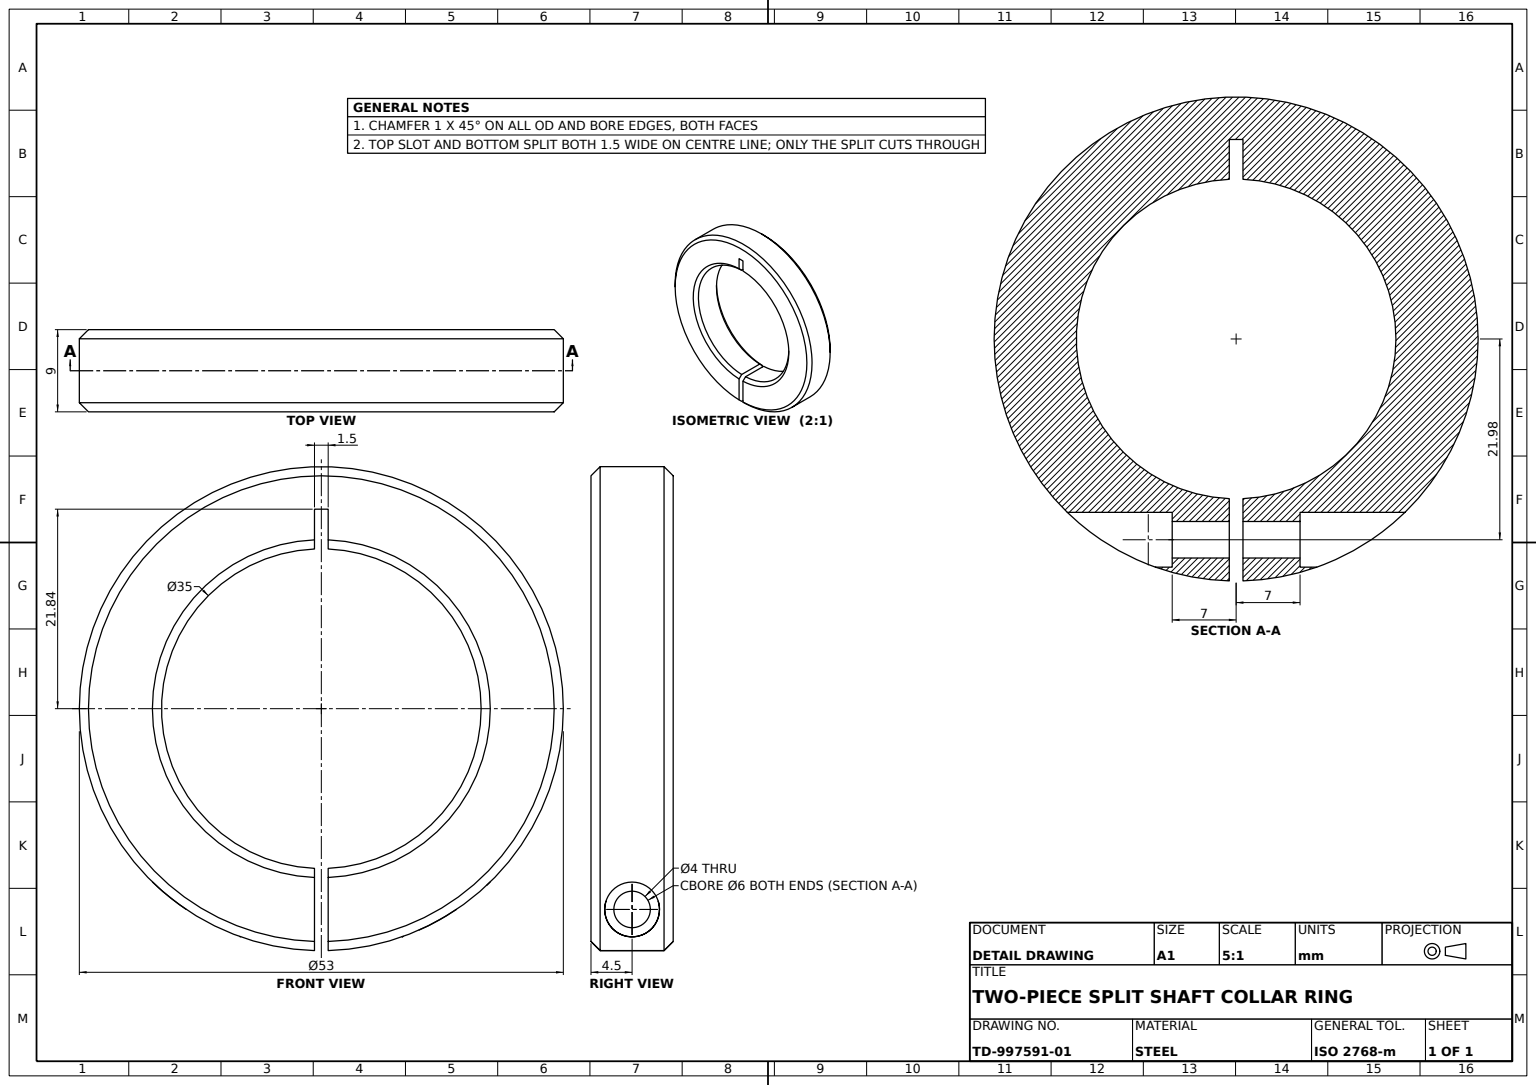
SolidWorks part; units mm, degrees
material "Plain Carbon Steel"
ref_plane "Front Plane" through (0, 0, 0) normal (0, 0, 1) x (1, 0, 0)
ref_plane "Top Plane" through (0, 0, 0) normal (0, 1, 0) x (1, 0, 0)
ref_plane "Right Plane" through (0, 0, 0) normal (1, 0, 0) x (0, 0, -1)
sketch "Ring Profile Sketch" plane through (0, 0, 0) normal (0, 0, 1) x (1, 0, 0)
  line L0 (0, 0) -> (14.8553, 0) construction
  line L1 (0, 0) -> (0, 37.451) construction
  line L2 (-0.75, 17.4839) -> (-0.75, 21.8439)
  line L3 (-0.75, 21.8439) -> (0.75, 21.8439)
  line L4 (0.75, 21.8439) -> (0.75, 17.4839)
  line L5 (0, 0) -> (0, -29.8508) construction
  line L6 (-0.75, -17.4839) -> (-0.75, -26.4894)
  line L8 (0.75, -26.4894) -> (0.75, -17.4839)
  arc A0 (-0.75, 17.4839) -> (-0.75, -17.4839) centre (0, 0) ccw
  arc A1 (0.75, -26.4894) -> (-0.75, -26.4894) centre (0, 0) ccw
  arc A2 (0.75, -17.4839) -> (0.75, 17.4839) centre (0, 0) ccw
  circle A3 centre (0, 0) radius 17.5 construction
  circle A5 centre (0, 0) radius 26.5 construction
  point P9 (16.7353, 5.1165)
  point P15 (26.5, 0)
  dimension "D1" = 35
  dimension "D6" = 4.36
  dimension "D3" = 1.5
  dimension "D4" = 0.75
  dimension "D5" = 0.75
  dimension "D2" = 9
extrude "Ring Body" add sketch "Ring Profile Sketch" along normal mid plane 9
chamfer "Edge Chamfer 1mm" distance 1 angle 45 6 edges at (-17.5, 0, -4.5) (17.5, 0, 4.5) (-17.5, 0, 4.5) (17.5, 0, -4.5) (0, 26.5, -4.5) (0, 26.5, 4.5)
sketch "Radial Cut Sketch" plane through (0, 0, 0) normal (1, 0, 0) x (0, 0, -1)
  line L0 (-4.5, 25.5) -> (-4.5, -25.489) construction
  line L1 (-3.5, -17.4839) -> (3.5, -17.4839) construction
  circle A0 centre (0, -21.9839) radius 2
  dimension "D2" = 4
  dimension "D1" = 4.5
  dimension "D3" = 4.5
extrude "Radial Cut" cut sketch "Radial Cut Sketch" against normal through all both and the other way through all
sketch "Slot Sketch" plane through (0, 0, 0) normal (1, 0, 0) x (0, 0, -1)
  circle A0 centre (0, -21.9839) radius 3
  dimension "D1" = 6
extrude "Slot Cut" cut sketch "Slot Sketch" along normal blind 25 from offset 7
mirror "Slot Mirror" about plane through (0, 0, 0) normal (1, 0, 0) of "Slot Cut"
